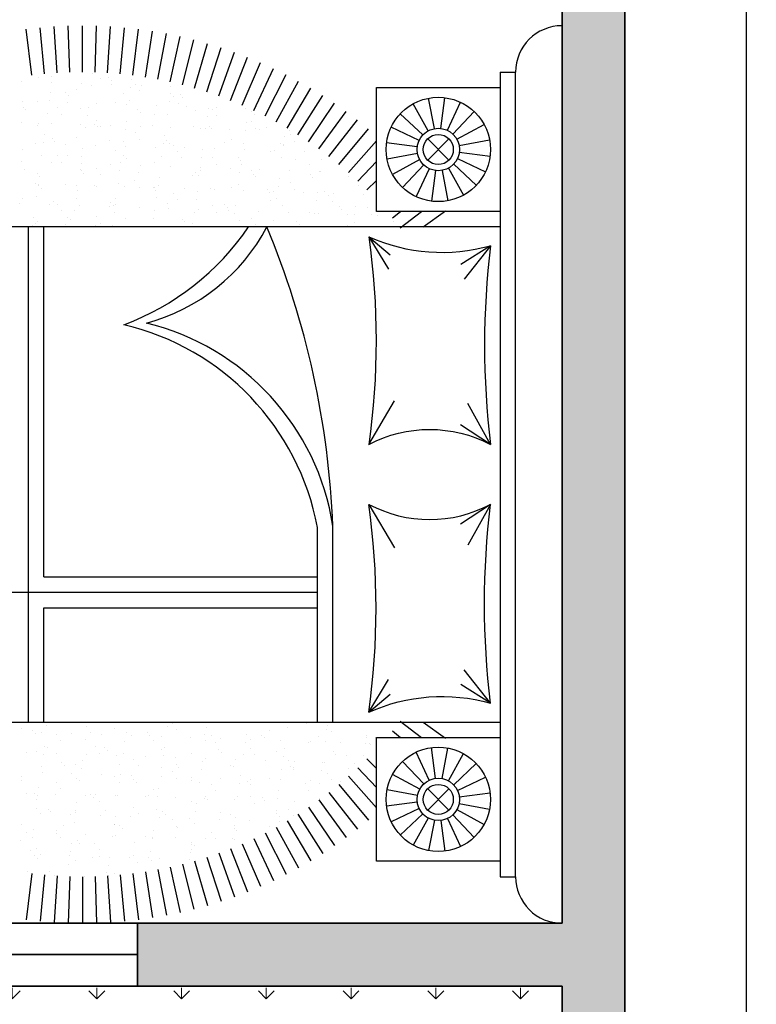
# Model space of a CAD drawing. Units: inches. Extents: x 1566 to 2546, y 1087 to 2705.
# Tile 5 of 27: x 1925 to 2018, y 1201 to 1326. Entities that reach past the tile are written whole.
import ezdxf

# ---------------------------------------------------------------- set-up
doc = ezdxf.new("R2010")
doc.units = ezdxf.units.IN
for name, color, linetype, lineweight in [('A-ANNO-DIMS', 2, 'Continuous', 18), ('A-FLOR-PATT', 3, 'Continuous', 13), ('A-FURN', 8, 'Continuous', 18), ('A-WALL', 7, 'Continuous', 35), ('A-WALL-PATT', 8, 'Continuous', 13)]:
    doc.layers.add(name, color=color, linetype=linetype, lineweight=lineweight)
for name, color, linetype in [('A-FRN', 11, 'Continuous'), ('A-HT', 15, 'Continuous'), ('L-HT', 1, 'Continuous')]:
    doc.layers.add(name, color=color, linetype=linetype)
doc.styles.get("Standard").update_dxf_attribs({"font": 'arial.ttf'})
doc.dimstyles.new('ISO-25', dxfattribs={"dimtxt": 2.5, "dimasz": 2.5, "dimexe": 1.25, "dimexo": 0.625, "dimtad": 1, "dimtxsty": 'Standard', "dimcen": 2.5, "dimadec": 0, "dimazin": 0, "dimtfac": 1, "dimtmove": 0, "dimatfit": 3, "dimfxl": 1, "dimarcsym": 0})

# ---------------------------------------------------------------- blocks, each defined once
blk = doc.blocks.new('*D7')
at = {"layer": 'A-ANNO-DIMS', "color": 0, "lineweight": -2, "transparency": 16777216}
for p, q in [((2002.15, 1778.2), (2018.24, 1778.2)), ((2016.99, 1156.7), (2016.99, 1775.7)), ((2002.15, 1154.2), (2018.24, 1154.2))]:
    blk.add_line(p, q, dxfattribs=at)
at = {"layer": 'A-ANNO-DIMS', "color": 0, "transparency": 16777216}
for points in [[(2016.58, 1775.7), (2017.41, 1775.7), (2016.99, 1778.2)], [(2016.58, 1156.7), (2017.41, 1156.7), (2016.99, 1154.2)]]:
    blk.add_solid(points, dxfattribs=at)
at = {"layer": 'Defpoints', "color": 0, "transparency": 16777216}
for p in [(2001.53, 1778.2), (2016.99, 1778.2), (2001.53, 1154.2)]:
    blk.add_point(p, dxfattribs=at)
at = {"layer": 'A-ANNO-DIMS', "color": 0, "transparency": 16777216, "insert": (2011.77, 1466.2), "char_height": 9, "attachment_point": 5, "rotation": 90}
blk.add_mtext("52'", dxfattribs=at)
blk = doc.blocks.new('*X21')
at = {"color": 0}
for p, q in [((1.1248, 1.7519), (1.1248, 1.7519)), ((3.1818, 1.75), (3.1818, 1.75)), ((0.731, 1.746), (0.731, 1.746)), ((0.7956, 1.742), (0.7956, 1.742)), ((0.813, 1.7413), (0.813, 1.7413)), ((0.8222, 1.7328), (0.8222, 1.7328)), ((0.8618, 1.7477), (0.8618, 1.7477)), ((0.9513, 1.7423), (0.9513, 1.7423)), ((0.9897, 1.747), (0.9897, 1.747)), ((1.016, 1.7368), (1.016, 1.7368)), ((1.107, 1.7426), (1.107, 1.7426)), ((2.8198, 1.7457), (2.8198, 1.7457)), ((2.8986, 1.7304), (2.8986, 1.7304)), ((2.9755, 1.7459), (2.9755, 1.7459)), ((2.988, 1.746), (2.988, 1.746)), ((3.0295, 1.7321), (3.0295, 1.7321)), ((3.1312, 1.7462), (3.1312, 1.7462)), ((3.1574, 1.7314), (3.1574, 1.7314)), ((3.2815, 1.7266), (3.2815, 1.7266)), ((0.7158, 1.6933), (0.7158, 1.6933)), ((0.7944, 1.6959), (0.7944, 1.6959)), ((0.8657, 1.693), (0.8657, 1.693)), ((0.8715, 1.6936), (0.8715, 1.6936)), ((0.9295, 1.7008), (0.9295, 1.7008)), ((1.0272, 1.6939), (1.0272, 1.6939)), ((1.0358, 1.6899), (1.0358, 1.6899)), ((1.0603, 1.7024), (1.0603, 1.7024)), ((1.0619, 1.6933), (1.0619, 1.6933)), ((1.0658, 1.6912), (1.0658, 1.6912)), ((1.1025, 1.6986), (1.1025, 1.6986)), ((1.1704, 1.7076), (1.1704, 1.7076)), ((1.1829, 1.6942), (1.1829, 1.6942)), ((1.1882, 1.7018), (1.1882, 1.7018)), ((1.1965, 1.711), (1.1965, 1.711)), ((2.8285, 1.7106), (2.8285, 1.7106)), ((2.8377, 1.7021), (2.8377, 1.7021)), ((2.8957, 1.6973), (2.8957, 1.6973)), ((3.0123, 1.6911), (3.0123, 1.6911)), ((3.0315, 1.7061), (3.0315, 1.7061)), ((3.0383, 1.6946), (3.0383, 1.6946)), ((3.0514, 1.6976), (3.0514, 1.6976)), ((3.079, 1.6999), (3.079, 1.6999)), ((3.1469, 1.7089), (3.1469, 1.7089)), ((3.1729, 1.7123), (3.1729, 1.7123)), ((3.2071, 1.6979), (3.2071, 1.6979)), ((3.2135, 1.7176), (3.2135, 1.7176)), ((3.228, 1.6868), (3.228, 1.6868)), ((3.2316, 1.7044), (3.2316, 1.7044)), ((3.2408, 1.696), (3.2408, 1.696)), ((0.7667, 1.6544), (0.7667, 1.6544)), ((0.7927, 1.6578), (0.7927, 1.6578)), ((0.8333, 1.6632), (0.8333, 1.6632)), ((0.9013, 1.6721), (0.9013, 1.6721)), ((0.9273, 1.6756), (0.9273, 1.6756)), ((0.9679, 1.6809), (0.9679, 1.6809)), ((1.075, 1.6828), (1.075, 1.6828)), ((1.1279, 1.6556), (1.1279, 1.6556)), ((2.8098, 1.6645), (2.8098, 1.6645)), ((2.8341, 1.6809), (2.8341, 1.6809)), ((2.8777, 1.6734), (2.8777, 1.6734)), ((2.8812, 1.6623), (2.8812, 1.6623)), ((2.9037, 1.6769), (2.9037, 1.6769)), ((2.9444, 1.6822), (2.9444, 1.6822)), ((2.962, 1.6803), (2.962, 1.6803)), ((3.0813, 1.6605), (3.0813, 1.6605)), ((3.0971, 1.6852), (3.0971, 1.6852)), ((3.2843, 1.6561), (3.2843, 1.6561)), ((0.7154, 1.6491), (0.7154, 1.6491)), ((0.7341, 1.6496), (0.7341, 1.6496)), ((0.8149, 1.6302), (0.8149, 1.6302)), ((0.865, 1.6513), (0.865, 1.6513)), ((0.9155, 1.6474), (0.9155, 1.6474)), ((0.9247, 1.6389), (0.9247, 1.6389)), ((0.9706, 1.6305), (0.9706, 1.6305)), ((0.9929, 1.6507), (0.9929, 1.6507)), ((1.1185, 1.6429), (1.1185, 1.6429)), ((1.1263, 1.6308), (1.1263, 1.6308)), ((2.8391, 1.6339), (2.8391, 1.6339)), ((2.9017, 1.634), (2.9017, 1.634)), ((2.9948, 1.6342), (2.9948, 1.6342)), ((3.0326, 1.6357), (3.0326, 1.6357)), ((3.0905, 1.6521), (3.0905, 1.6521)), ((3.1505, 1.6345), (3.1505, 1.6345)), ((3.1605, 1.6351), (3.1605, 1.6351)), ((3.2956, 1.64), (3.2956, 1.64)), ((0.7652, 1.6035), (0.7652, 1.6035)), ((0.7744, 1.595), (0.7744, 1.595)), ((0.7976, 1.5996), (0.7976, 1.5996)), ((0.836, 1.6168), (0.836, 1.6168)), ((0.9326, 1.6044), (0.9326, 1.6044)), ((0.9682, 1.599), (0.9682, 1.599)), ((0.9917, 1.6171), (0.9917, 1.6171)), ((1.0635, 1.6061), (1.0635, 1.6061)), ((1.1474, 1.6173), (1.1474, 1.6173)), ((1.1683, 1.5973), (1.1683, 1.5973)), ((1.1914, 1.6055), (1.1914, 1.6055)), ((2.8602, 1.6205), (2.8602, 1.6205)), ((2.931, 1.6167), (2.931, 1.6167)), ((2.9402, 1.6082), (2.9402, 1.6082)), ((3.0159, 1.6207), (3.0159, 1.6207)), ((3.134, 1.6122), (3.134, 1.6122)), ((3.1716, 1.621), (3.1716, 1.621)), ((3.2596, 1.5943), (3.2596, 1.5943)), ((0.7562, 1.5681), (0.7562, 1.5681)), ((0.9119, 1.5684), (0.9119, 1.5684)), ((1.0676, 1.5687), (1.0676, 1.5687)), ((1.0819, 1.5665), (1.0819, 1.5665)), ((1.108, 1.5699), (1.108, 1.5699)), ((1.1311, 1.5592), (1.1311, 1.5592)), ((1.1486, 1.5753), (1.1486, 1.5753)), ((1.1775, 1.5889), (1.1775, 1.5889)), ((2.8373, 1.5846), (2.8373, 1.5846)), ((2.9361, 1.5721), (2.9361, 1.5721)), ((2.9652, 1.584), (2.9652, 1.584)), ((2.9837, 1.5683), (2.9837, 1.5683)), ((3.0584, 1.5678), (3.0584, 1.5678)), ((3.0844, 1.5712), (3.0844, 1.5712)), ((3.0918, 1.5724), (3.0918, 1.5724)), ((3.1002, 1.5888), (3.1002, 1.5888)), ((3.1251, 1.5765), (3.1251, 1.5765)), ((3.1838, 1.5666), (3.1838, 1.5666)), ((3.193, 1.5855), (3.193, 1.5855)), ((3.219, 1.5889), (3.219, 1.5889)), ((3.2311, 1.5905), (3.2311, 1.5905)), ((3.2475, 1.5727), (3.2475, 1.5727)), ((0.7373, 1.5533), (0.7373, 1.5533)), ((0.8128, 1.531), (0.8128, 1.531)), ((0.8179, 1.5552), (0.8179, 1.5552)), ((0.8388, 1.5345), (0.8388, 1.5345)), ((0.8681, 1.555), (0.8681, 1.555)), ((0.8794, 1.5398), (0.8794, 1.5398)), ((0.9474, 1.5488), (0.9474, 1.5488)), ((0.9734, 1.5522), (0.9734, 1.5522)), ((0.996, 1.5544), (0.996, 1.5544)), ((1.014, 1.5575), (1.014, 1.5575)), ((1.018, 1.5534), (1.018, 1.5534)), ((1.0272, 1.545), (1.0272, 1.545)), ((2.8152, 1.5357), (2.8152, 1.5357)), ((2.8559, 1.5411), (2.8559, 1.5411)), ((2.9049, 1.5377), (2.9049, 1.5377)), ((2.9238, 1.55), (2.9238, 1.55)), ((2.9498, 1.5535), (2.9498, 1.5535)), ((2.9905, 1.5588), (2.9905, 1.5588)), ((3.0358, 1.5394), (3.0358, 1.5394)), ((3.1637, 1.5388), (3.1637, 1.5388)), ((3.193, 1.5582), (3.193, 1.5582)), ((3.2987, 1.5436), (3.2987, 1.5436)), ((0.7042, 1.5167), (0.7042, 1.5167)), ((0.7448, 1.5221), (0.7448, 1.5221)), ((0.8007, 1.5032), (0.8007, 1.5032)), ((0.8553, 1.505), (0.8553, 1.505)), ((0.8677, 1.5096), (0.8677, 1.5096)), ((0.8769, 1.5011), (0.8769, 1.5011)), ((0.9358, 1.5081), (0.9358, 1.5081)), ((1.011, 1.5053), (1.011, 1.5053)), ((1.0666, 1.5098), (1.0666, 1.5098)), ((1.0707, 1.5051), (1.0707, 1.5051)), ((1.1667, 1.5056), (1.1667, 1.5056)), ((1.1945, 1.5091), (1.1945, 1.5091)), ((2.8334, 1.5245), (2.8334, 1.5245)), ((2.8795, 1.5087), (2.8795, 1.5087)), ((3.0334, 1.5227), (3.0334, 1.5227)), ((3.0352, 1.509), (3.0352, 1.509)), ((3.0427, 1.5143), (3.0427, 1.5143)), ((3.0563, 1.4955), (3.0563, 1.4955)), ((3.1909, 1.5093), (3.1909, 1.5093)), ((3.212, 1.4958), (3.212, 1.4958)), ((3.2365, 1.5183), (3.2365, 1.5183)), ((0.7174, 1.4657), (0.7174, 1.4657)), ((0.7207, 1.4913), (0.7207, 1.4913)), ((0.8764, 1.4916), (0.8764, 1.4916)), ((1.0321, 1.4919), (1.0321, 1.4919)), ((1.1878, 1.4921), (1.1878, 1.4921)), ((2.8404, 1.4882), (2.8404, 1.4882)), ((2.8831, 1.4789), (2.8831, 1.4789)), ((2.8924, 1.4704), (2.8924, 1.4704)), ((2.9006, 1.4953), (2.9006, 1.4953)), ((2.9683, 1.4876), (2.9683, 1.4876)), ((3.0862, 1.4744), (3.0862, 1.4744)), ((3.1034, 1.4925), (3.1034, 1.4925)), ((3.2343, 1.4942), (3.2343, 1.4942)), ((3.2651, 1.4655), (3.2651, 1.4655)), ((3.2862, 1.4727), (3.2862, 1.4727)), ((3.2954, 1.4643), (3.2954, 1.4643)), ((0.7266, 1.4572), (0.7266, 1.4572)), ((0.7404, 1.457), (0.7404, 1.457)), ((0.7966, 1.4429), (0.7966, 1.4429)), ((0.8713, 1.4586), (0.8713, 1.4586)), ((0.9204, 1.4613), (0.9204, 1.4613)), ((0.9523, 1.4432), (0.9523, 1.4432)), ((0.9992, 1.458), (0.9992, 1.458)), ((1.0601, 1.4341), (1.0601, 1.4341)), ((1.108, 1.4435), (1.108, 1.4435)), ((1.1205, 1.4595), (1.1205, 1.4595)), ((1.128, 1.4431), (1.128, 1.4431)), ((1.1297, 1.4511), (1.1297, 1.4511)), ((1.1342, 1.4629), (1.1342, 1.4629)), ((1.1541, 1.4465), (1.1541, 1.4465)), ((1.1947, 1.4519), (1.1947, 1.4519)), ((2.8208, 1.4466), (2.8208, 1.4466)), ((2.908, 1.4414), (2.908, 1.4414)), ((2.9765, 1.4469), (2.9765, 1.4469)), ((3.0366, 1.4354), (3.0366, 1.4354)), ((3.0389, 1.443), (3.0389, 1.443)), ((3.1045, 1.4444), (3.1045, 1.4444)), ((3.1305, 1.4478), (3.1305, 1.4478)), ((3.1322, 1.4472), (3.1322, 1.4472)), ((3.1668, 1.4424), (3.1668, 1.4424)), ((3.1712, 1.4532), (3.1712, 1.4532)), ((3.2391, 1.4621), (3.2391, 1.4621)), ((3.2879, 1.4475), (3.2879, 1.4475)), ((0.7701, 1.4174), (0.7701, 1.4174)), ((0.8039, 1.4069), (0.8039, 1.4069)), ((0.8589, 1.4076), (0.8589, 1.4076)), ((0.8849, 1.4111), (0.8849, 1.4111)), ((0.9255, 1.4164), (0.9255, 1.4164)), ((0.9389, 1.4118), (0.9389, 1.4118)), ((0.9701, 1.4157), (0.9701, 1.4157)), ((0.9794, 1.4072), (0.9794, 1.4072)), ((0.9935, 1.4254), (0.9935, 1.4254)), ((1.0195, 1.4288), (1.0195, 1.4288)), ((1.0698, 1.4134), (1.0698, 1.4134)), ((1.1732, 1.4112), (1.1732, 1.4112)), ((1.1977, 1.4128), (1.1977, 1.4128)), ((2.8353, 1.4089), (2.8353, 1.4089)), ((2.8613, 1.4124), (2.8613, 1.4124)), ((2.902, 1.4177), (2.902, 1.4177)), ((2.9359, 1.4306), (2.9359, 1.4306)), ((2.9699, 1.4267), (2.9699, 1.4267)), ((2.9959, 1.4301), (2.9959, 1.4301)), ((3.1359, 1.4288), (3.1359, 1.4288)), ((3.1451, 1.4204), (3.1451, 1.4204)), ((0.7243, 1.3899), (0.7243, 1.3899)), ((0.74, 1.3795), (0.74, 1.3795)), ((0.7503, 1.3934), (0.7503, 1.3934)), ((0.7909, 1.3987), (0.7909, 1.3987)), ((0.8198, 1.3718), (0.8198, 1.3718)), ((0.8957, 1.3798), (0.8957, 1.3798)), ((1.0514, 1.3801), (1.0514, 1.3801)), ((2.8436, 1.3919), (2.8436, 1.3919)), ((2.9199, 1.3835), (2.9199, 1.3835)), ((2.9409, 1.37), (2.9409, 1.37)), ((2.9715, 1.3913), (2.9715, 1.3913)), ((2.9856, 1.385), (2.9856, 1.385)), ((2.9948, 1.3765), (2.9948, 1.3765)), ((3.0756, 1.3838), (3.0756, 1.3838)), ((3.0967, 1.3703), (3.0967, 1.3703)), ((3.1065, 1.3961), (3.1065, 1.3961)), ((3.1886, 1.3805), (3.1886, 1.3805)), ((3.2313, 1.384), (3.2313, 1.384)), ((3.2374, 1.3978), (3.2374, 1.3978)), ((3.2524, 1.3706), (3.2524, 1.3706)), ((0.7436, 1.3606), (0.7436, 1.3606)), ((0.761, 1.3661), (0.761, 1.3661)), ((0.8291, 1.3633), (0.8291, 1.3633)), ((0.8744, 1.3623), (0.8744, 1.3623)), ((0.9168, 1.3664), (0.9168, 1.3664)), ((1.0023, 1.3617), (1.0023, 1.3617)), ((1.0229, 1.3673), (1.0229, 1.3673)), ((1.0725, 1.3667), (1.0725, 1.3667)), ((1.1374, 1.3665), (1.1374, 1.3665)), ((2.8353, 1.3411), (2.8353, 1.3411)), ((2.9112, 1.345), (2.9112, 1.345)), ((3.0383, 1.3367), (3.0383, 1.3367)), ((3.0421, 1.3467), (3.0421, 1.3467)), ((3.17, 1.3461), (3.17, 1.3461)), ((0.807, 1.3105), (0.807, 1.3105)), ((0.837, 1.3177), (0.837, 1.3177)), ((0.8726, 1.3235), (0.8726, 1.3235)), ((0.9421, 1.3154), (0.9421, 1.3154)), ((0.9927, 1.318), (0.9927, 1.318)), ((1.0656, 1.3054), (1.0656, 1.3054)), ((1.0726, 1.3217), (1.0726, 1.3217)), ((1.0729, 1.3171), (1.0729, 1.3171)), ((1.0818, 1.3133), (1.0818, 1.3133)), ((1.1062, 1.3108), (1.1062, 1.3108)), ((1.1484, 1.3183), (1.1484, 1.3183)), ((1.1741, 1.3197), (1.1741, 1.3197)), ((2.8445, 1.3326), (2.8445, 1.3326)), ((2.8611, 1.3214), (2.8611, 1.3214)), ((3.0169, 1.3217), (3.0169, 1.3217)), ((3.042, 1.3067), (3.042, 1.3067)), ((3.0827, 1.312), (3.0827, 1.312)), ((3.1506, 1.321), (3.1506, 1.321)), ((3.1726, 1.322), (3.1726, 1.322)), ((3.1766, 1.3244), (3.1766, 1.3244)), ((3.2173, 1.3298), (3.2173, 1.3298)), ((3.2384, 1.3349), (3.2384, 1.3349)), ((3.2476, 1.3265), (3.2476, 1.3265)), ((0.837, 1.2753), (0.837, 1.2753)), ((0.905, 1.2843), (0.905, 1.2843)), ((0.9223, 1.2779), (0.9223, 1.2779)), ((0.931, 1.2877), (0.931, 1.2877)), ((0.9716, 1.293), (0.9716, 1.293)), ((1.0396, 1.302), (1.0396, 1.302)), ((1.1253, 1.2734), (1.1253, 1.2734)), ((2.8135, 1.2766), (2.8135, 1.2766)), ((2.8467, 1.2956), (2.8467, 1.2956)), ((2.8814, 1.2855), (2.8814, 1.2855)), ((2.888, 1.2928), (2.888, 1.2928)), ((2.9074, 1.289), (2.9074, 1.289)), ((2.9481, 1.2943), (2.9481, 1.2943)), ((2.9746, 1.2949), (2.9746, 1.2949)), ((3.016, 1.3033), (3.016, 1.3033)), ((3.0881, 1.291), (3.0881, 1.291)), ((3.0973, 1.2826), (3.0973, 1.2826)), ((3.1097, 1.2998), (3.1097, 1.2998)), ((3.2406, 1.3015), (3.2406, 1.3015)), ((0.7467, 1.2643), (0.7467, 1.2643)), ((0.7704, 1.2665), (0.7704, 1.2665)), ((0.7803, 1.2543), (0.7803, 1.2543)), ((0.7964, 1.27), (0.7964, 1.27)), ((0.8014, 1.2409), (0.8014, 1.2409)), ((0.8776, 1.2659), (0.8776, 1.2659)), ((0.9315, 1.2694), (0.9315, 1.2694)), ((0.936, 1.2546), (0.936, 1.2546)), ((0.9571, 1.2412), (0.9571, 1.2412)), ((1.0055, 1.2653), (1.0055, 1.2653)), ((1.0918, 1.2549), (1.0918, 1.2549)), ((1.1128, 1.2414), (1.1128, 1.2414)), ((1.1405, 1.2702), (1.1405, 1.2702)), ((2.8045, 1.258), (2.8045, 1.258)), ((2.8256, 1.2446), (2.8256, 1.2446)), ((2.9143, 1.2487), (2.9143, 1.2487)), ((2.9378, 1.2472), (2.9378, 1.2472)), ((2.9602, 1.2583), (2.9602, 1.2583)), ((2.9813, 1.2448), (2.9813, 1.2448)), ((3.0452, 1.2503), (3.0452, 1.2503)), ((3.1159, 1.2586), (3.1159, 1.2586)), ((3.137, 1.2451), (3.137, 1.2451)), ((3.1408, 1.2427), (3.1408, 1.2427)), ((3.1731, 1.2497), (3.1731, 1.2497)), ((0.772, 1.234), (0.772, 1.234)), ((0.7812, 1.2255), (0.7812, 1.2255)), ((0.8102, 1.2142), (0.8102, 1.2142)), ((0.9452, 1.2191), (0.9452, 1.2191)), ((0.975, 1.2296), (0.975, 1.2296)), ((1.0761, 1.2207), (1.0761, 1.2207)), ((1.1751, 1.2278), (1.1751, 1.2278)), ((1.1843, 1.2194), (1.1843, 1.2194)), ((2.947, 1.2387), (2.947, 1.2387)), ((0.8247, 1.1857), (0.8247, 1.1857)), ((0.8773, 1.1925), (0.8773, 1.1925)), ((1.0248, 1.184), (1.0248, 1.184)), ((1.033, 1.1928), (1.033, 1.1928)), ((1.0857, 1.1786), (1.0857, 1.1786)), ((1.1117, 1.182), (1.1117, 1.182)), ((1.1523, 1.1874), (1.1523, 1.1874)), ((1.1887, 1.1931), (1.1887, 1.1931)), ((2.8499, 1.1992), (2.8499, 1.1992)), ((2.9015, 1.1962), (2.9015, 1.1962)), ((2.9778, 1.1986), (2.9778, 1.1986)), ((2.9905, 1.1989), (2.9905, 1.1989)), ((3.0572, 1.1965), (3.0572, 1.1965)), ((3.0621, 1.1799), (3.0621, 1.1799)), ((3.0881, 1.1833), (3.0881, 1.1833)), ((3.1128, 1.2035), (3.1128, 1.2035)), ((3.1288, 1.1887), (3.1288, 1.1887)), ((3.1906, 1.1971), (3.1906, 1.1971)), ((3.1967, 1.1976), (3.1967, 1.1976)), ((3.1998, 1.1887), (3.1998, 1.1887)), ((3.2129, 1.1968), (3.2129, 1.1968)), ((3.2227, 1.201), (3.2227, 1.201)), ((3.2437, 1.2051), (3.2437, 1.2051)), ((0.8425, 1.1466), (0.8425, 1.1466)), ((0.8807, 1.1696), (0.8807, 1.1696)), ((0.8831, 1.1519), (0.8831, 1.1519)), ((0.9511, 1.1609), (0.9511, 1.1609)), ((0.9771, 1.1643), (0.9771, 1.1643)), ((1.0086, 1.169), (1.0086, 1.169)), ((1.0177, 1.1696), (1.0177, 1.1696)), ((1.034, 1.1755), (1.034, 1.1755)), ((1.1437, 1.1739), (1.1437, 1.1739)), ((2.8189, 1.1479), (2.8189, 1.1479)), ((2.8402, 1.155), (2.8402, 1.155)), ((2.8596, 1.1532), (2.8596, 1.1532)), ((2.9175, 1.1523), (2.9175, 1.1523)), ((2.9275, 1.1622), (2.9275, 1.1622)), ((2.9535, 1.1656), (2.9535, 1.1656)), ((2.9942, 1.1709), (2.9942, 1.1709)), ((3.0403, 1.1533), (3.0403, 1.1533)), ((3.0484, 1.154), (3.0484, 1.154)), ((3.1763, 1.1534), (3.1763, 1.1534)), ((0.8133, 1.1179), (0.8133, 1.1179)), ((0.8165, 1.1432), (0.8165, 1.1432)), ((0.8207, 1.1291), (0.8207, 1.1291)), ((0.8418, 1.1157), (0.8418, 1.1157)), ((0.8745, 1.1401), (0.8745, 1.1401)), ((0.8837, 1.1316), (0.8837, 1.1316)), ((0.9484, 1.1227), (0.9484, 1.1227)), ((0.9764, 1.1294), (0.9764, 1.1294)), ((0.9975, 1.116), (0.9975, 1.116)), ((1.0775, 1.1356), (1.0775, 1.1356)), ((1.0792, 1.1244), (1.0792, 1.1244)), ((1.1321, 1.1297), (1.1321, 1.1297)), ((1.1532, 1.1162), (1.1532, 1.1162)), ((2.8449, 1.1328), (2.8449, 1.1328)), ((2.866, 1.1194), (2.866, 1.1194)), ((3.0006, 1.1331), (3.0006, 1.1331)), ((3.0217, 1.1196), (3.0217, 1.1196)), ((3.0495, 1.1448), (3.0495, 1.1448)), ((3.1563, 1.1334), (3.1563, 1.1334)), ((3.1774, 1.1199), (3.1774, 1.1199)), ((0.9272, 1.0918), (0.9272, 1.0918)), ((1.1273, 1.09), (1.1273, 1.09)), ((2.853, 1.1029), (2.853, 1.1029)), ((2.89, 1.1094), (2.89, 1.1094)), ((2.8992, 1.1009), (2.8992, 1.1009)), ((2.9809, 1.1023), (2.9809, 1.1023)), ((3.093, 1.105), (3.093, 1.105)), ((3.116, 1.1071), (3.116, 1.1071)), ((0.8839, 1.0733), (0.8839, 1.0733)), ((0.9177, 1.0673), (0.9177, 1.0673)), ((1.0118, 1.0727), (1.0118, 1.0727)), ((1.0734, 1.0676), (1.0734, 1.0676)), ((1.1318, 1.0552), (1.1318, 1.0552)), ((1.1365, 1.0816), (1.1365, 1.0816)), ((1.1468, 1.0775), (1.1468, 1.0775)), ((1.1578, 1.0586), (1.1578, 1.0586)), ((1.1984, 1.064), (1.1984, 1.064)), ((2.9206, 1.056), (2.9206, 1.056)), ((2.9419, 1.071), (2.9419, 1.071)), ((2.9427, 1.0611), (2.9427, 1.0611)), ((3.0515, 1.0577), (3.0515, 1.0577)), ((3.0976, 1.0713), (3.0976, 1.0713)), ((3.1082, 1.0565), (3.1082, 1.0565)), ((3.1342, 1.0599), (3.1342, 1.0599)), ((3.1428, 1.0594), (3.1428, 1.0594)), ((3.152, 1.0509), (3.152, 1.0509)), ((3.1749, 1.0653), (3.1749, 1.0653)), ((3.1794, 1.057), (3.1794, 1.057)), ((0.8165, 1.0215), (0.8165, 1.0215)), ((0.8626, 1.0198), (0.8626, 1.0198)), ((0.8886, 1.0232), (0.8886, 1.0232)), ((0.9292, 1.0285), (0.9292, 1.0285)), ((0.9515, 1.0264), (0.9515, 1.0264)), ((0.977, 1.0462), (0.977, 1.0462)), ((0.9862, 1.0377), (0.9862, 1.0377)), ((0.9972, 1.0375), (0.9972, 1.0375)), ((1.0232, 1.0409), (1.0232, 1.0409)), ((1.0638, 1.0463), (1.0638, 1.0463)), ((1.0824, 1.0281), (1.0824, 1.0281)), ((1.18, 1.0417), (1.18, 1.0417)), ((2.839, 1.0211), (2.839, 1.0211)), ((2.865, 1.0245), (2.865, 1.0245)), ((2.9057, 1.0298), (2.9057, 1.0298)), ((2.9736, 1.0388), (2.9736, 1.0388)), ((2.9996, 1.0422), (2.9996, 1.0422)), ((3.0403, 1.0475), (3.0403, 1.0475)), ((0.8267, 1.0023), (0.8267, 1.0023)), ((0.8359, 0.9938), (0.8359, 0.9938)), ((0.8611, 1.0039), (0.8611, 1.0039)), ((0.8822, 0.9905), (0.8822, 0.9905)), ((1.0168, 1.0042), (1.0168, 1.0042)), ((1.0297, 0.9979), (1.0297, 0.9979)), ((1.0379, 0.9908), (1.0379, 0.9908)), ((1.1725, 1.0045), (1.1725, 1.0045)), ((1.1936, 0.991), (1.1936, 0.991)), ((2.8562, 1.0065), (2.8562, 1.0065)), ((2.8853, 1.0076), (2.8853, 1.0076)), ((2.9064, 0.9942), (2.9064, 0.9942)), ((2.9841, 1.0059), (2.9841, 1.0059)), ((2.9925, 1.0155), (2.9925, 1.0155)), ((3.0017, 1.007), (3.0017, 1.007)), ((3.041, 1.0079), (3.041, 1.0079)), ((3.0621, 0.9944), (3.0621, 0.9944)), ((3.1191, 1.0108), (3.1191, 1.0108)), ((0.887, 0.9769), (0.887, 0.9769)), ((1.0149, 0.9763), (1.0149, 0.9763)), ((1.15, 0.9812), (1.15, 0.9812)), ((2.8421, 0.9716), (2.8421, 0.9716)), ((2.8514, 0.9631), (2.8514, 0.9631)), ((2.9238, 0.9597), (2.9238, 0.9597)), ((3.0452, 0.9672), (3.0452, 0.9672)), ((3.0547, 0.9613), (3.0547, 0.9613)), ((0.8794, 0.954), (0.8794, 0.954)), ((0.9546, 0.93), (0.9546, 0.93)), ((0.9581, 0.9421), (0.9581, 0.9421)), ((1.0795, 0.9523), (1.0795, 0.9523)), ((1.0855, 0.9317), (1.0855, 0.9317)), ((1.0887, 0.9438), (1.0887, 0.9438)), ((1.1099, 0.9229), (1.1099, 0.9229)), ((1.1138, 0.9424), (1.1138, 0.9424)), ((1.1779, 0.9318), (1.1779, 0.9318)), ((2.8266, 0.9455), (2.8266, 0.9455)), ((2.8949, 0.9233), (2.8949, 0.9233)), ((2.9823, 0.9458), (2.9823, 0.9458)), ((3.0864, 0.9242), (3.0864, 0.9242)), ((3.138, 0.9461), (3.138, 0.9461)), ((0.9087, 0.8964), (0.9087, 0.8964)), ((0.9292, 0.9084), (0.9292, 0.9084)), ((0.9347, 0.8998), (0.9347, 0.8998)), ((0.9384, 0.8999), (0.9384, 0.8999)), ((0.9753, 0.9052), (0.9753, 0.9052)), ((1.0433, 0.9141), (1.0433, 0.9141)), ((1.0693, 0.9175), (1.0693, 0.9175)), ((1.1322, 0.904), (1.1322, 0.904)), ((2.8593, 0.9102), (2.8593, 0.9102)), ((2.8851, 0.8977), (2.8851, 0.8977)), ((2.9111, 0.9011), (2.9111, 0.9011)), ((2.9518, 0.9064), (2.9518, 0.9064)), ((2.9872, 0.9096), (2.9872, 0.9096)), ((3.0197, 0.9154), (3.0197, 0.9154)), ((3.0457, 0.9188), (3.0457, 0.9188)), ((3.0949, 0.9216), (3.0949, 0.9216)), ((3.1041, 0.9131), (3.1041, 0.9131)), ((3.1223, 0.9144), (3.1223, 0.9144)), ((0.8902, 0.8806), (0.8902, 0.8806)), ((0.9015, 0.8787), (0.9015, 0.8787)), ((0.9226, 0.8653), (0.9226, 0.8653)), ((0.9819, 0.8601), (0.9819, 0.8601)), ((1.0181, 0.88), (1.0181, 0.88)), ((1.0572, 0.879), (1.0572, 0.879)), ((1.0783, 0.8655), (1.0783, 0.8655)), ((1.1531, 0.8848), (1.1531, 0.8848)), ((2.8172, 0.8887), (2.8172, 0.8887)), ((2.9257, 0.8824), (2.9257, 0.8824)), ((2.9269, 0.8633), (2.9269, 0.8633)), ((2.9446, 0.8777), (2.9446, 0.8777)), ((2.9468, 0.8689), (2.9468, 0.8689)), ((2.9538, 0.8692), (2.9538, 0.8692)), ((3.0578, 0.865), (3.0578, 0.865)), ((3.0814, 0.8827), (3.0814, 0.8827)), ((3.1025, 0.8692), (3.1025, 0.8692)), ((0.9578, 0.8337), (0.9578, 0.8337)), ((1.0887, 0.8354), (1.0887, 0.8354)), ((1.1819, 0.8583), (1.1819, 0.8583)), ((1.1912, 0.8499), (1.1912, 0.8499)), ((2.9973, 0.8294), (2.9973, 0.8294)), ((0.9985, 0.8169), (0.9985, 0.8169)), ((1.0316, 0.8145), (1.0316, 0.8145)), ((1.0409, 0.806), (1.0409, 0.806)), ((1.1542, 0.8172), (1.1542, 0.8172)), ((1.156, 0.7995), (1.156, 0.7995)), ((2.8035, 0.8253), (2.8035, 0.8253)), ((2.8625, 0.8138), (2.8625, 0.8138)), ((2.867, 0.8203), (2.867, 0.8203)), ((2.9904, 0.8132), (2.9904, 0.8132)), ((3.0227, 0.8206), (3.0227, 0.8206)), ((0.9808, 0.7764), (0.9808, 0.7764)), ((1.0212, 0.7836), (1.0212, 0.7836)), ((1.0214, 0.7818), (1.0214, 0.7818)), ((1.0844, 0.7662), (1.0844, 0.7662)), ((1.0894, 0.7907), (1.0894, 0.7907)), ((1.1154, 0.7941), (1.1154, 0.7941)), ((1.1563, 0.7885), (1.1563, 0.7885)), ((2.847, 0.7855), (2.847, 0.7855)), ((2.8633, 0.7653), (2.8633, 0.7653)), ((2.9301, 0.767), (2.9301, 0.767)), ((2.9312, 0.7743), (2.9312, 0.7743)), ((2.9572, 0.7777), (2.9572, 0.7777)), ((2.9979, 0.7831), (2.9979, 0.7831)), ((3.0471, 0.7838), (3.0471, 0.7838)), ((1.0918, 0.739), (1.0918, 0.739)), ((1.0976, 0.7538), (1.0976, 0.7538)), ((1.1187, 0.7403), (1.1187, 0.7403)), ((2.8104, 0.7569), (2.8104, 0.7569)), ((2.8227, 0.76), (2.8227, 0.76)), ((2.8314, 0.7435), (2.8314, 0.7435)), ((2.8968, 0.7399), (2.8968, 0.7399)), ((2.9661, 0.7572), (2.9661, 0.7572)), ((2.9871, 0.7437), (2.9871, 0.7437)), ((1.1341, 0.7206), (1.1341, 0.7206)), ((1.1433, 0.7121), (1.1433, 0.7121)), ((2.8656, 0.7175), (2.8656, 0.7175)), ((2.906, 0.7314), (2.906, 0.7314)), ((2.9935, 0.7169), (2.9935, 0.7169)), ((1.0389, 0.6917), (1.0389, 0.6917)), ((1.1594, 0.6922), (1.1594, 0.6922)), ((1.1615, 0.6707), (1.1615, 0.6707)), ((1.1868, 0.6723), (1.1868, 0.6723)), ((1.1946, 0.692), (1.1946, 0.692)), ((2.9073, 0.6951), (2.9073, 0.6951)), ((2.9332, 0.6706), (2.9332, 0.6706)), ((2.9495, 0.6916), (2.9495, 0.6916)), ((1.0675, 0.6584), (1.0675, 0.6584)), ((1.095, 0.6427), (1.095, 0.6427)), ((1.1355, 0.6673), (1.1355, 0.6673)), ((2.8688, 0.6366), (2.8688, 0.6366)), ((2.9094, 0.6419), (2.9094, 0.6419)), ((1.138, 0.6286), (1.138, 0.6286)), ((1.159, 0.6151), (1.159, 0.6151)), ((2.8427, 0.6332), (2.8427, 0.6332)), ((2.8507, 0.6317), (2.8507, 0.6317)), ((2.8688, 0.6212), (2.8688, 0.6212)), ((2.8718, 0.6183), (2.8718, 0.6183)), ((1.1626, 0.5958), (1.1626, 0.5958)), ((2.849, 0.6021), (2.849, 0.6021)), ((1.1816, 0.5439), (1.1816, 0.5439)), ((2.8013, 0.5694), (2.8013, 0.5694))]:
    blk.add_line(p, q, dxfattribs=at)
blk = doc.blocks.new('A$C6796526C')
at = {"layer": 'A-FRN'}
for p, q in [((0, 3), (2.9, 3)), ((2.75, 2.85), (0.15, 2.85)), ((0.15, 2.8), (0.15, 2.85)), ((2.75, 2.8), (2.75, 2.85)), ((0.15, 2.8), (2.75, 2.8)), ((0.2, 2.4), (0.2, 2.8)), ((0.6, 2.8), (0.6, 2.4)), ((2.3, 2.4), (2.3, 2.8)), ((2.7, 2.8), (2.7, 2.4)), ((0.6, 2.4), (0.2, 2.4)), ((2.7, 2.4), (2.3, 2.4))]:
    blk.add_line(p, q, dxfattribs=at)
blk.add_lwpolyline([(0.65, 2.8), (0.65, 0.9), (2.25, 0.9), (2.25, 2.8)], dxfattribs=at)
for points in [[(0.6821, 2.3755, 0.175461), (0.7109, 2.7686)], [(0.7109, 2.7686, 0.059544), (1.3533, 2.7686)], [(1.3533, 2.3755, -0.248743), (1.3533, 2.7686)], [(2.1891, 2.7686, -0.059544), (1.5467, 2.7686)], [(1.5467, 2.3755, 0.248743), (1.5467, 2.7686)], [(2.2179, 2.3755, -0.175461), (2.1891, 2.7686)], [(0.6821, 2.3755, -0.069628), (1.3533, 2.3755)], [(2.2179, 2.3755, 0.069628), (1.5467, 2.3755)], [(2.25, 2.2594), (1.6173, 2.2594, 0.303651), (0.9607, 1.6568, 0.210515), (0.65, 2.0462)]]:
    blk.add_lwpolyline(points, format="xyb", dxfattribs=at)
for centre, radius in [((0.4, 2.6), 0.1686), ((2.5, 2.6), 0.1686), ((0.4, 2.6), 0.0686), ((2.5, 2.6), 0.0686)]:
    blk.add_circle(centre, radius, dxfattribs=at)
for centre, radius, start, end in [((0.15, 3), 0.15, 180, 270), ((2.75, 3), 0.15, 270, 0), ((1.7313, -0.5592), 2.8209, 92.3174, 112.5397)]:
    blk.add_arc(centre, radius, start, end, dxfattribs=at)
at = {"layer": 'A-HT'}
for p, q in [((0.65, 2.5511), (0.5977, 2.6231)), ((2.25, 2.5511), (2.3023, 2.6231)), ((0.6532, 2.4772), (0.6, 2.5458)), ((2.2468, 2.4772), (2.3, 2.5458)), ((0.6213, 2.4517), (0.6, 2.4775)), ((2.2787, 2.4517), (2.3, 2.4775)), ((0.4749, 2.3097), (0.3724, 2.4)), ((0.5023, 2.3399), (0.4384, 2.4)), ((0.5308, 2.3692), (0.5, 2.4)), ((2.3692, 2.3692), (2.4, 2.4)), ((2.3977, 2.3399), (2.4616, 2.4)), ((2.4251, 2.3097), (2.5276, 2.4)), ((0.4483, 2.2787), (0.3328, 2.3743)), ((2.4517, 2.2787), (2.5672, 2.3743)), ((0.4228, 2.2468), (0.3043, 2.3387)), ((2.4772, 2.2468), (2.5957, 2.3387)), ((0.3983, 2.2141), (0.2769, 2.3023)), ((2.5017, 2.2141), (2.6231, 2.3023)), ((0.3748, 2.1807), (0.2507, 2.265)), ((2.5252, 2.1807), (2.6493, 2.265)), ((0.3524, 2.1466), (0.2257, 2.2269)), ((2.5476, 2.1466), (2.6743, 2.2269)), ((0.331, 2.1118), (0.2019, 2.1881)), ((2.569, 2.1118), (2.6981, 2.1881)), ((0.3108, 2.0763), (0.1794, 2.1485)), ((2.5892, 2.0763), (2.7206, 2.1485)), ((0.2917, 2.0402), (0.158, 2.1083)), ((2.6083, 2.0402), (2.742, 2.1083)), ((0.2737, 2.0035), (0.138, 2.0674)), ((2.6263, 2.0035), (2.762, 2.0674)), ((0.2569, 1.9663), (0.1193, 2.0259)), ((2.6431, 1.9663), (2.7807, 2.0259)), ((0.2413, 1.9286), (0.1018, 1.9838)), ((2.6587, 1.9286), (2.7982, 1.9838)), ((0.2269, 1.8904), (0.0857, 1.9412)), ((2.6731, 1.8904), (2.8143, 1.9412)), ((0.2136, 1.8517), (0.071, 1.8981)), ((2.6864, 1.8517), (2.829, 1.8981)), ((0.2016, 1.8127), (0.0576, 1.8545)), ((2.6984, 1.8127), (2.8424, 1.8545)), ((0.1908, 1.7733), (0.0456, 1.8106)), ((2.7092, 1.7733), (2.8544, 1.8106)), ((0.1813, 1.7336), (0.0349, 1.7663)), ((2.7187, 1.7336), (2.8651, 1.7663)), ((0.173, 1.6936), (0.0257, 1.7217)), ((2.727, 1.6936), (2.8743, 1.7217)), ((0.166, 1.6534), (0.0179, 1.6768)), ((2.734, 1.6534), (2.8821, 1.6768)), ((0.1603, 1.6129), (0.0114, 1.6317)), ((2.7397, 1.6129), (2.8886, 1.6317)), ((0.1558, 1.5723), (0.0064, 1.5865)), ((2.7442, 1.5723), (2.8936, 1.5865)), ((0.1526, 1.5316), (0.0029, 1.541)), ((2.7474, 1.5316), (2.8971, 1.541)), ((0.1506, 1.4908), (0.0007, 1.4955)), ((2.7494, 1.4908), (2.8993, 1.4955)), ((0.15, 1.45), (0, 1.45)), ((2.75, 1.45), (2.9, 1.45)), ((0.1506, 1.4092), (0.0007, 1.4045)), ((2.7494, 1.4092), (2.8993, 1.4045)), ((0.1526, 1.3684), (0.0029, 1.359)), ((2.7474, 1.3684), (2.8971, 1.359)), ((0.1558, 1.3277), (0.0064, 1.3135)), ((2.7442, 1.3277), (2.8936, 1.3135)), ((0.1603, 1.2871), (0.0114, 1.2683)), ((2.7397, 1.2871), (2.8886, 1.2683))]:
    blk.add_line(p, q, dxfattribs=at)
at = {"layer": 'L-HT'}
for p, q in [((0.7109, 2.7686), (0.8188, 2.6839)), ((0.7109, 2.7686), (0.7717, 2.6727)), ((1.3533, 2.7686), (1.2212, 2.6952)), ((1.3533, 2.7686), (1.2893, 2.6715)), ((1.5467, 2.7686), (1.6107, 2.6715)), ((1.5467, 2.7686), (1.6788, 2.6952)), ((2.1891, 2.7686), (2.0812, 2.6839)), ((2.1891, 2.7686), (2.1283, 2.6727)), ((0.3671, 2.6601), (0.319, 2.7478)), ((0.3873, 2.6674), (0.3687, 2.7656)), ((0.4087, 2.668), (0.4214, 2.7672)), ((0.4293, 2.662), (0.472, 2.7524)), ((2.4707, 2.662), (2.428, 2.7524)), ((2.4913, 2.668), (2.4786, 2.7672)), ((2.5127, 2.6674), (2.5313, 2.7656)), ((2.5329, 2.6601), (2.581, 2.7478)), ((0.3501, 2.647), (0.2773, 2.7156)), ((0.447, 2.6499), (0.5156, 2.7227)), ((2.453, 2.6499), (2.3844, 2.7227)), ((2.5499, 2.647), (2.6227, 2.7156)), ((0.4601, 2.6329), (0.5478, 2.681)), ((2.4399, 2.6329), (2.3522, 2.681)), ((0.338, 2.6293), (0.2476, 2.672)), ((2.562, 2.6293), (2.6524, 2.672)), ((0.332, 2.6087), (0.2328, 2.6214)), ((0.3657, 2.5657), (0.4343, 2.6343)), ((0.4343, 2.5657), (0.3657, 2.6343)), ((0.4674, 2.6127), (0.5656, 2.6313)), ((2.4326, 2.6127), (2.3344, 2.6313)), ((2.4657, 2.5657), (2.5343, 2.6343)), ((2.5343, 2.5657), (2.4657, 2.6343)), ((2.568, 2.6087), (2.6672, 2.6214)), ((0.3326, 2.5873), (0.2344, 2.5687)), ((0.468, 2.5913), (0.5672, 2.5786)), ((2.432, 2.5913), (2.3328, 2.5786)), ((2.5674, 2.5873), (2.6656, 2.5687)), ((0.3399, 2.5671), (0.2522, 2.519)), ((0.353, 2.5501), (0.2844, 2.4773)), ((0.4499, 2.553), (0.5227, 2.4844)), ((0.462, 2.5707), (0.5524, 2.528)), ((2.438, 2.5707), (2.3476, 2.528)), ((2.4501, 2.553), (2.3773, 2.4844)), ((2.547, 2.5501), (2.6156, 2.4773)), ((2.5601, 2.5671), (2.6478, 2.519)), ((0.3707, 2.538), (0.328, 2.4476)), ((0.3913, 2.532), (0.3786, 2.4328)), ((0.4127, 2.5326), (0.4313, 2.4344)), ((0.4329, 2.5399), (0.481, 2.4522)), ((2.4671, 2.5399), (2.419, 2.4522)), ((2.4873, 2.5326), (2.4687, 2.4344)), ((2.5087, 2.532), (2.5214, 2.4328)), ((2.5293, 2.538), (2.572, 2.4476)), ((1.3533, 2.3755), (1.2125, 2.4585)), ((1.5467, 2.3755), (1.6875, 2.4585)), ((0.6821, 2.3755), (0.7405, 2.4447)), ((0.6821, 2.3755), (0.7872, 2.4395)), ((2.2179, 2.3755), (2.1128, 2.4395)), ((2.2179, 2.3755), (2.1595, 2.4447)), ((2.25, 2.2094), (1.6212, 2.2094)), ((1.7809, 1.3249), (1.7809, 2.2094)), ((1.8309, 0.9), (1.8309, 2.2094)), ((1.8809, 1.3249), (1.8809, 2.2094)), ((1.7809, 1.3249), (0.65, 1.3249)), ((2.25, 1.3249), (1.8809, 1.3249)), ((0.65, 1.2749), (2.25, 1.2749))]:
    blk.add_line(p, q, dxfattribs=at)
for centre in [(0.4, 2.6), (2.5, 2.6)]:
    blk.add_circle(centre, 0.0486, dxfattribs=at)
for centre, radius, start, end in [((1.7721, 1.396), 0.8272, 100.5107, 166.872), ((0.1786, 1.2908), 0.8406, 20.4105, 55.8901)]:
    blk.add_arc(centre, radius, start, end, dxfattribs=at)
at = {"layer": 'A-HT', "extrusion": (0, 0, -1), "zscale": -1, "rotation": 180}
blk.add_blockref('*X21', (0.55, 3), dxfattribs=at)

msp = doc.modelspace()

# ---------------------------------------------------------------- hatches: boundary and pattern name
at = {"layer": 'A-FLOR-PATT'}
h = msp.add_hatch(dxfattribs=at)
h.set_pattern_fill('GRASS', color=256, scale=0.3)
h.paths.add_polyline_path([(1745.53, 1270.2), (1645.53, 1270.2), (1645.53, 1159.2), (1745.53, 1159.2)])
h.paths.add_polyline_path([(1993.53, 1203.2), (1819.53, 1203.2), (1819.53, 1155.2), (1993.53, 1155.2)])
h.paths.add_polyline_path([(1667.62, 1196.42), (1716.72, 1196.42), (1716.72, 1222.54), (1667.62, 1222.54)], flags=24)
h.paths.add_polyline_path([(1881.06, 1171.45), (1935.47, 1171.45), (1935.47, 1197.57), (1881.06, 1197.57)], flags=24)
at = {"layer": 'A-WALL-PATT'}
h = msp.add_hatch(color=256, dxfattribs=at)
h.dxf.hatch_style = 1
h.paths.add_polyline_path([(2001.53, 1778.2), (1641.53, 1778.2), (1641.53, 1746.2), (1649.53, 1746.2), (1649.53, 1770.2), (1769.53, 1770.2), (1769.53, 1650.2), (1767.53, 1650.2), (1767.53, 1648.2), (1767.53, 1646.2), (1819.53, 1646.2), (1819.53, 1650.2), (1773.53, 1650.2), (1773.53, 1770.2), (1941.53, 1770.2), (1941.53, 1756.2), (1945.53, 1756.2), (1945.53, 1770.2), (1993.53, 1770.2), (1993.53, 1650.2), (1945.53, 1650.2), (1945.53, 1652.2), (1943.53, 1652.2), (1941.53, 1652.2), (1941.53, 1650.2), (1867.53, 1650.2), (1867.53, 1642.2), (1871.53, 1642.2), (1871.53, 1646.2), (1993.53, 1646.2), (1993.53, 1526.2), (1871.53, 1526.2), (1871.53, 1606.2), (1867.53, 1606.2), (1867.53, 1522.2), (1993.53, 1522.2), (1993.53, 1387.2), (1959.53, 1387.2), (1959.53, 1397.2), (1955.53, 1397.2), (1955.53, 1387.2), (1903.53, 1387.2), (1903.53, 1383.2), (1993.53, 1383.2), (1993.53, 1364.3), (1993.53, 1211.2), (1939.53, 1211.2), (1939.53, 1203.2), (1993.53, 1203.2), (1993.53, 1154.2), (2001.53, 1154.2)])
h.paths.add_polyline_path([(1649.53, 1646.2), (1731.53, 1646.2), (1731.53, 1650.2), (1649.53, 1650.2), (1649.53, 1674.2), (1641.53, 1674.2), (1641.53, 1622.2), (1649.53, 1622.2)], flags=17)
h.paths.add_polyline_path([(1649.53, 1550.2), (1641.53, 1550.2), (1641.53, 1510.2), (1649.53, 1510.2), (1649.53, 1522.2), (1731.53, 1522.2), (1731.53, 1500.2), (1735.53, 1500.2), (1735.53, 1522.2), (1767.53, 1522.2), (1767.53, 1500.2), (1771.53, 1500.2), (1771.53, 1526.2), (1649.53, 1526.2)], flags=17)
h.paths.add_polyline_path([(1649.53, 1464.2), (1735.53, 1464.2), (1735.53, 1470.2), (1731.53, 1470.2), (1731.53, 1468.2), (1649.53, 1468.2), (1649.53, 1480.2), (1641.53, 1480.2), (1641.53, 1419.2), (1649.53, 1419.2)], flags=17)
h.paths.add_polyline_path([(1649.53, 1323.2), (1641.53, 1323.2), (1641.53, 1270.2), (1667.53, 1270.2), (1667.53, 1278.2), (1649.53, 1278.2)], flags=17)
h.paths.add_polyline_path([(1763.53, 1278.2), (1727.53, 1278.2), (1727.53, 1270.2), (1763.53, 1270.2)], flags=17)
h.paths.add_polyline_path([(1823.53, 1383.2), (1827.53, 1383.2), (1827.53, 1385.2), (1827.53, 1387.2), (1819.53, 1387.2), (1819.53, 1324.21), (1819.53, 1278.2), (1811.53, 1278.2), (1811.53, 1274.2), (1811.53, 1270.2), (1819.53, 1270.2), (1819.53, 1203.2), (1877.53, 1203.2), (1877.53, 1211.2), (1823.53, 1211.2)], flags=17)

# ---------------------------------------------------------------- linework, layer by layer
at = {"layer": 'A-WALL'}
for p, q in [((2001.53, 1778.2), (2001.53, 1154.2)), ((1993.53, 1383.2), (1993.53, 1211.2)), ((1823.53, 1211.2), (1993.53, 1211.2)), ((1939.53, 1211.2), (1939.53, 1203.2)), ((1939.53, 1211.2), (1939.53, 1203.2)), ((1877.53, 1207.2), (1939.53, 1207.2)), ((1877.53, 1207.2), (1939.53, 1207.2)), ((1819.53, 1203.2), (1993.53, 1203.2)), ((1993.53, 1203.2), (1993.53, 1154.2))]:
    msp.add_line(p, q, dxfattribs=at)

# ---------------------------------------------------------------- block references
at = {"layer": 'A-FURN', "xscale": 39.3701, "yscale": 39.3701, "zscale": 39.3701, "rotation": 270}
msp.add_blockref('A$C6796526C', (1875.42, 1325.37), dxfattribs=at)

# ---------------------------------------------------------------- dimensions: what is measured, and where the dimension line sits
at = {"layer": 'A-ANNO-DIMS'}
dim = msp.add_linear_dim(base=(2016.99, 1778.2), p1=(2001.53, 1154.2), p2=(2001.53, 1778.2), angle=90, dimstyle='ISO-25', override={"dimtxt": 9, "dimdec": 1, "dimlunit": 3, "dimclrd": 0, "dimclre": 0, "dimclrt": 0, "dimtdec": 1}, dxfattribs=at)
dim.commit()
dim.dimension.update_dxf_attribs({"geometry": '*D7', "text_midpoint": (2011.77, 1466.2)})

doc.saveas('drawing.dxf')
